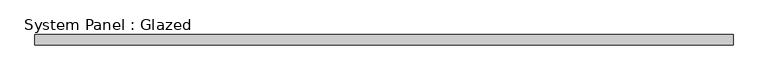
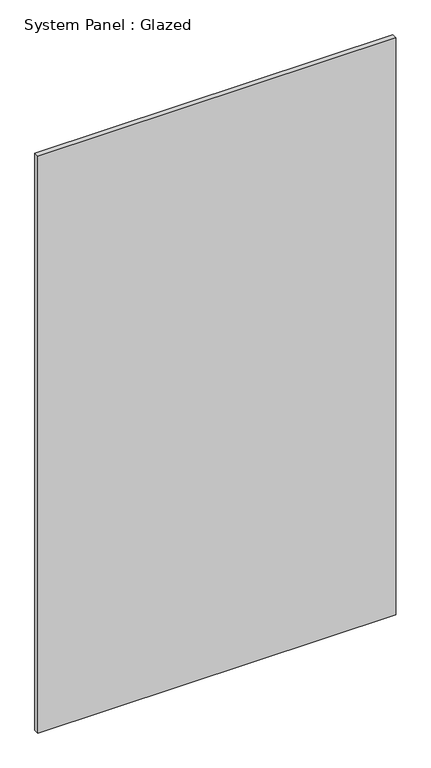
"""IFC4 building model written with IfcOpenShell, lengths in millimetres: plate geometry, System Panel : Glazed."""

from ifc_helpers import new_model, si_unit, origin, origin_with_axes, place, context, project, spatial, polyline, outline, extrude, source, transform, mapped, element, save


def system_panel_glazed_baea53c3(model_context):
    return source(origin(), model_context, "Body", "SweptSolid", [
        extrude(outline(polyline([(857.25, 19.05), (-857.25, 19.05), (-857.25, 44.45), (857.25, 44.45), (857.25, 19.05)])), origin_with_axes(), (0.0, 0.0, 1.0), 2921.0),
    ])


if __name__ == "__main__":
    model = new_model("IFC4")
    model_context = context("Model", 3, world=origin())
    ifc_project = project(units=[si_unit("LENGTHUNIT", "METRE", prefix="MILLI")], contexts=[model_context])
    site = spatial("IfcSite", under=ifc_project)
    building = spatial("IfcBuilding", under=site)
    placement = place(None, origin())
    system_panel_glazed_shape = system_panel_glazed_baea53c3(model_context)
    element("IfcPlate", 1, ObjectType="System Panel : Glazed", at=placement, inside=building, context=model_context, shape_type="MappedRepresentation", body=[
        mapped(system_panel_glazed_shape, transform((0.0, 0.0, 0.0), x_axis=(1.0, 0.0, 0.0), y_axis=(0.0, 1.0, 0.0), z_axis=(0.0, 0.0, 1.0))),
    ])
    save(model, "model.ifc")

# Revit data of these elements
# Type "System Panel : Glazed"
#   Construction Type Id = "GSP4R"
#   Analytic Construction = "1/8 in Pilkington single glazing"
#   Visual Light Transmittance = 0.9
#   Solar Heat Gain Coefficient = 0.86
#   Heat Transfer Coefficient (U) = 1.18115 BTU/(h·ft²·°F)
# Element 1 (IfcPlate, "System Panel : Glazed")
#   Materials on its faces: "Glass"
# Materials
#   "Glass": class "Glass", colour RGB 0 128 192, transparency 0.75, Description = "Soda Lime Glass", Cost = 0
